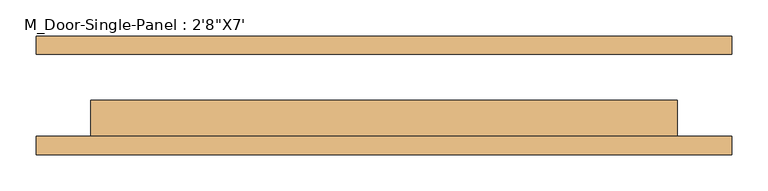
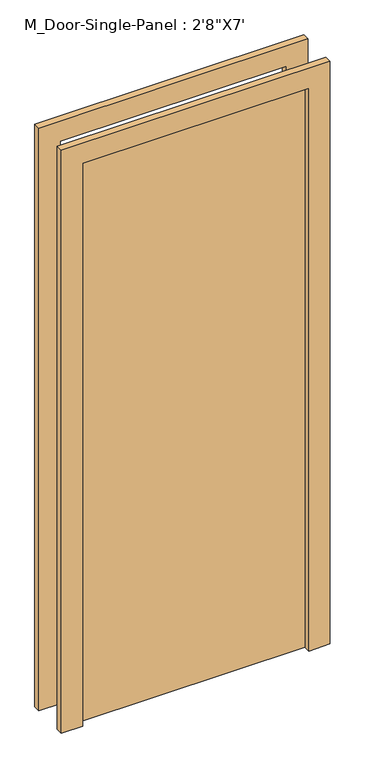
"""IFC4 building model written with IfcOpenShell, lengths in millimetres: door geometry."""

from ifc_helpers import new_model, si_unit, frame, origin, origin_with_axes, place, context, project, spatial, polyline, outline, extrude, source, transform, mapped, element, save


def door_82def9da(model_context):
    return source(origin(), model_context, "Body", "SweptSolid", [
        extrude(outline(polyline([(406.4, -7.15), (406.4, -57.15), (-406.4, -57.15), (-406.4, -7.15), (406.4, -7.15)])), origin_with_axes(), (0.0, 0.0, 1.0), 2133.6),
        extrude(outline(polyline([(2209.8, 482.6), (2209.8, -482.6), (0.0, -482.6), (0.0, -406.4), (2133.6, -406.4), (2133.6, 406.4), (0.0, 406.4), (0.0, 482.6), (2209.8, 482.6)])), frame((0.0, 57.15, 0.0), z_axis=(0.0, 1.0, 0.0), x_axis=(0.0, 0.0, 1.0)), (0.0, 0.0, 1.0), 25.0),
        extrude(outline(polyline([(2209.8, -482.6), (0.0, -482.6), (0.0, -406.4), (2133.6, -406.4), (2133.6, 406.4), (0.0, 406.4), (0.0, 482.6), (2209.8, 482.6), (2209.8, -482.6)])), frame((0.0, -82.15, 0.0), z_axis=(0.0, 1.0, 0.0), x_axis=(0.0, 0.0, 1.0)), (0.0, 0.0, 1.0), 25.0),
    ])


if __name__ == "__main__":
    model = new_model("IFC4")
    model_context = context("Model", 3, world=origin())
    ifc_project = project(units=[si_unit("LENGTHUNIT", "METRE", prefix="MILLI")], contexts=[model_context])
    site = spatial("IfcSite", under=ifc_project)
    building = spatial("IfcBuilding", under=site)
    placement = place(None, origin())
    door_shape = door_82def9da(model_context)
    element("IfcDoor", 1, ObjectType="M_Door-Single-Panel : 2'8\"X7'", at=placement, inside=building, context=model_context, shape_type="MappedRepresentation", body=[
        mapped(door_shape, transform((0.0, 0.0, 0.0), x_axis=(1.0, 0.0, 0.0), y_axis=(0.0, 1.0, 0.0), z_axis=(0.0, 0.0, 1.0))),
    ])
    save(model, "model.ifc")

# Revit data of these elements
# Type "M_Door-Single-Panel : 2'8\"X7'"
#   Type Mark = "9"
#   Construction Type Id = "DOOR"
#   Assembly Code = "C1020300"
#   Analytic Construction = "Wooden"
#   Thickness = 0' - 1.9685"
#   Thermal Resistance (R) = 2.5876 (h·ft²·°F)/BTU
#   Swing Angle [instance default] = 90.00°
#   Heat Transfer Coefficient (U) = 0.3865 BTU/(h·ft²·°F)
#   Height = 7' - 0"
#   Trim Projection Ext = 0' - 0.98425"
#   Trim Projection Int = 0' - 0.98425"
#   Trim Width = 0' - 3.14961"
#   Width = 2' - 8"
#   Define Thermal Properties by = 1
#   Panel Material = Wood - Birch - Solid Stained Light Low Gloss
#   Trim Material = Paint - Sienna
#   Visual Light Transmittance = 0
#   Solar Heat Gain Coefficient = 0
#   Function = (empty or 0)
#   Wall Closure = (empty or 0)
# Element 1 (IfcDoor, "M_Door-Single-Panel : 2'8\"X7'")
#   Materials on its faces: "Paint - Sienna", "Wood - Birch - Solid Stained Light Low Gloss"
# Materials
#   "Wood - Birch - Solid Stained Light Low Gloss": class "Wood", colour RGB 210 159 95, transparency 0, Cost = 0
#   "Paint - Sienna": colour RGB 118 70 51, transparency 0, Cost = 0
